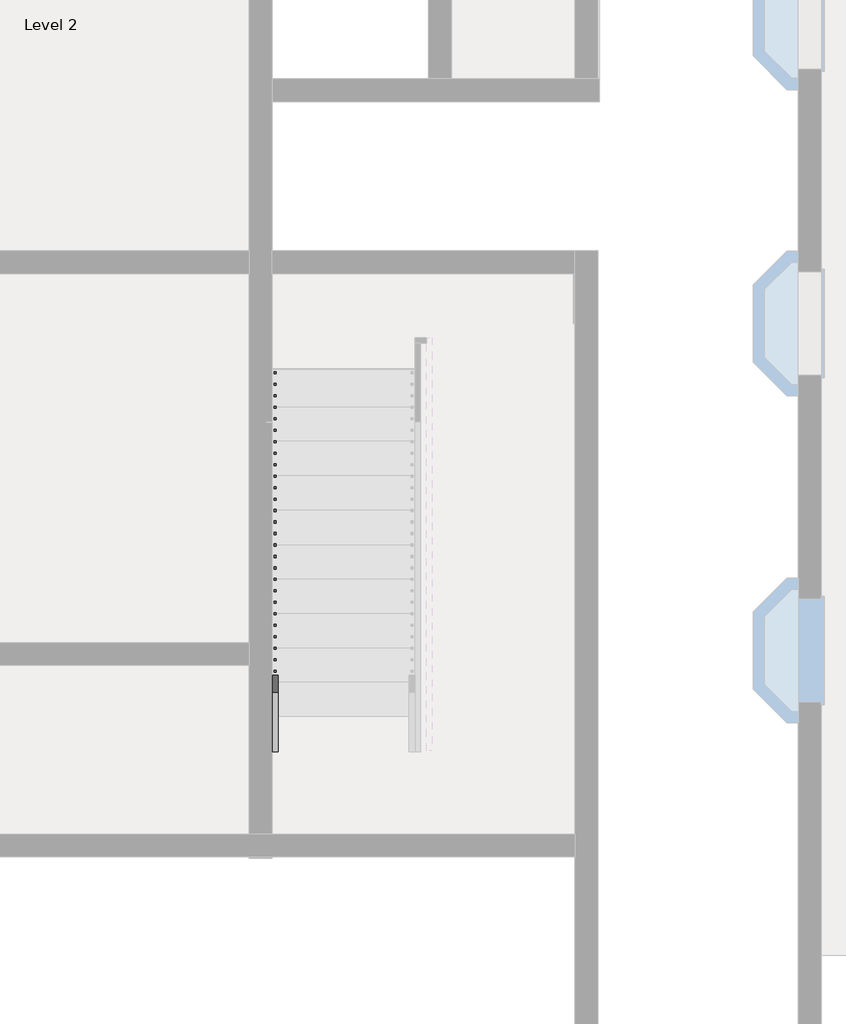
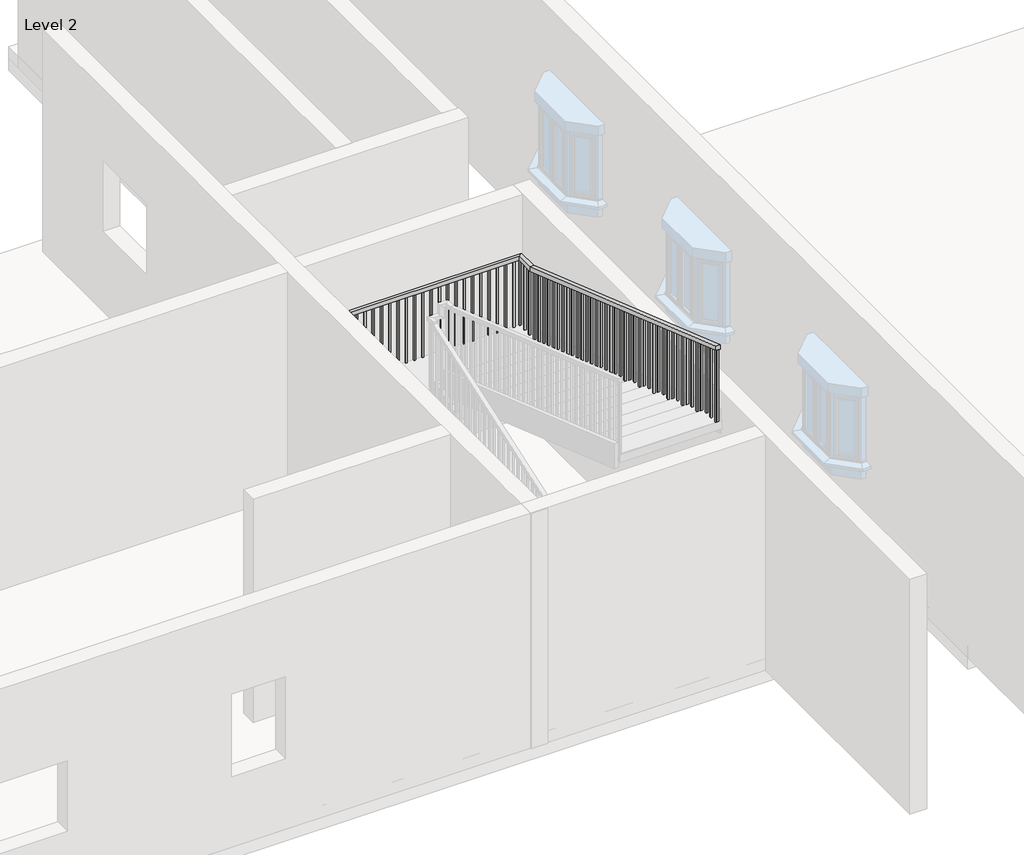
# One storey, part 8 of 14: 1 railing.
"""IFC4 building model written with IfcOpenShell, lengths in millimetres."""

from ifc_helpers import new_model, si_unit, frame, origin, place, context, project, spatial, polyline, outline, extrude, faceted_brep, element, save

model = new_model("IFC4")

# Units and contexts
model_context = context("Model", 3, world=origin())
ifc_project = project(units=[si_unit("LENGTHUNIT", "METRE", prefix="MILLI")], contexts=[model_context])

# Site, building, storey
site = spatial("IfcSite", under=ifc_project)
building = spatial("IfcBuilding", under=site)
storey = spatial("IfcBuildingStorey", under=building, Name="Level 2", Elevation=3048.0)

# Railing
placement = place(None, origin())
element("IfcRailing", 1, ObjectType="Handrail - Rectangular", at=placement, inside=storey, context=model_context, shape_type="SolidModel", body=[
    faceted_brep([(-3857.687215, -9955.5916506, 4067.9076923), (-3857.687215, -9955.5916506, 4014.1602476), (-3806.887215, -9955.5916506, 4014.1602476), (-3806.887215, -9955.5916506, 4067.9076923), (-3857.687215, -6291.6416506, 5334.0), (-3857.687215, -6283.1120276, 5283.2), (-3806.887215, -6283.1120276, 5283.2), (-3806.887215, -6291.6416506, 5334.0), (-3857.687215, -5713.7916506, 5334.0), (-3857.687215, -5713.7916506, 5283.2), (-3806.887215, -5764.5916506, 5283.2), (-3806.887215, -5764.5916506, 5334.0), (-1190.687215, -5713.7916506, 5334.0), (-1190.687215, -5713.7916506, 5283.2), (-1241.487215, -5764.5916506, 5283.2), (-1241.487215, -5764.5916506, 5334.0), (-1190.687215, -5986.8416506, 5334.0), (-1190.687215, -5995.3852679, 5283.2), (-1241.487215, -5995.3852679, 5283.2), (-1241.487215, -5986.8416506, 5334.0), (-1190.687215, -9949.2416506, 6705.6), (-1241.487215, -9949.2416506, 6705.6), (-1241.487215, -9949.2416506, 6651.842594), (-1190.687215, -9949.2416506, 6651.842594)], [[[0, 1, 2, 3]], [[1, 0, 4, 5]], [[2, 1, 5, 6]], [[3, 2, 6, 7]], [[0, 3, 7, 4]], [[5, 4, 8, 9]], [[6, 5, 9, 10]], [[7, 6, 10, 11]], [[4, 7, 11, 8]], [[9, 8, 12, 13]], [[10, 9, 13, 14]], [[11, 10, 14, 15]], [[8, 11, 15, 12]], [[13, 12, 16, 17]], [[14, 13, 17, 18]], [[15, 14, 18, 19]], [[12, 15, 19, 16]], [[20, 21, 22, 23]], [[17, 16, 20, 23]], [[18, 17, 23, 22]], [[19, 18, 22, 21]], [[16, 19, 21, 20]]]),
    extrude(outline(polyline([(-9895.2666506, 6633.1589402), (-9895.2666506, 5685.6923077), (-9914.3166506, 5685.6923077), (-9914.3166506, 6639.7531709), (-9895.2666506, 6633.1589402)])), frame((-1225.612215, 0.0, 0.0), z_axis=(1.0, 0.0, 0.0), x_axis=(0.0, 1.0, 0.0)), (0.0, 0.0, 1.0), 19.05),
    extrude(outline(polyline([(-9793.6666506, 6597.9897094), (-9793.6666506, 5685.6923077), (-9812.7166506, 5685.6923077), (-9812.7166506, 6604.5839402), (-9793.6666506, 6597.9897094)])), frame((-1225.612215, 0.0, 0.0), z_axis=(1.0, 0.0, 0.0), x_axis=(0.0, 1.0, 0.0)), (0.0, 0.0, 1.0), 19.05),
    extrude(outline(polyline([(-9692.0666506, 6562.8204786), (-9692.0666506, 5685.6923077), (-9711.1166506, 5685.6923077), (-9711.1166506, 6569.4147094), (-9692.0666506, 6562.8204786)])), frame((-1225.612215, 0.0, 0.0), z_axis=(1.0, 0.0, 0.0), x_axis=(0.0, 1.0, 0.0)), (0.0, 0.0, 1.0), 19.05),
    extrude(outline(polyline([(-9590.4666506, 6527.6512479), (-9590.4666506, 5580.1846154), (-9609.5166506, 5580.1846154), (-9609.5166506, 6534.2454786), (-9590.4666506, 6527.6512479)])), frame((-1225.612215, 0.0, 0.0), z_axis=(1.0, 0.0, 0.0), x_axis=(0.0, 1.0, 0.0)), (0.0, 0.0, 1.0), 19.05),
    extrude(outline(polyline([(-9488.8666506, 6492.4820171), (-9488.8666506, 5580.1846154), (-9507.9166506, 5580.1846154), (-9507.9166506, 6499.0762479), (-9488.8666506, 6492.4820171)])), frame((-1225.612215, 0.0, 0.0), z_axis=(1.0, 0.0, 0.0), x_axis=(0.0, 1.0, 0.0)), (0.0, 0.0, 1.0), 19.05),
    extrude(outline(polyline([(-9387.2666506, 6457.3127863), (-9387.2666506, 5580.1846154), (-9406.3166506, 5580.1846154), (-9406.3166506, 6463.9070171), (-9387.2666506, 6457.3127863)])), frame((-1225.612215, 0.0, 0.0), z_axis=(1.0, 0.0, 0.0), x_axis=(0.0, 1.0, 0.0)), (0.0, 0.0, 1.0), 19.05),
    extrude(outline(polyline([(-9285.6666506, 6422.1435556), (-9285.6666506, 5474.6769231), (-9304.7166506, 5474.6769231), (-9304.7166506, 6428.7377863), (-9285.6666506, 6422.1435556)])), frame((-1225.612215, 0.0, 0.0), z_axis=(1.0, 0.0, 0.0), x_axis=(0.0, 1.0, 0.0)), (0.0, 0.0, 1.0), 19.05),
    extrude(outline(polyline([(-9184.0666506, 6386.9743248), (-9184.0666506, 5474.6769231), (-9203.1166506, 5474.6769231), (-9203.1166506, 6393.5685556), (-9184.0666506, 6386.9743248)])), frame((-1225.612215, 0.0, 0.0), z_axis=(1.0, 0.0, 0.0), x_axis=(0.0, 1.0, 0.0)), (0.0, 0.0, 1.0), 19.05),
    extrude(outline(polyline([(-9082.4666506, 6351.805094), (-9082.4666506, 5474.6769231), (-9101.5166506, 5474.6769231), (-9101.5166506, 6358.3993248), (-9082.4666506, 6351.805094)])), frame((-1225.612215, 0.0, 0.0), z_axis=(1.0, 0.0, 0.0), x_axis=(0.0, 1.0, 0.0)), (0.0, 0.0, 1.0), 19.05),
    extrude(outline(polyline([(-8980.8666506, 6316.6358632), (-8980.8666506, 5369.1692308), (-8999.9166506, 5369.1692308), (-8999.9166506, 6323.230094), (-8980.8666506, 6316.6358632)])), frame((-1225.612215, 0.0, 0.0), z_axis=(1.0, 0.0, 0.0), x_axis=(0.0, 1.0, 0.0)), (0.0, 0.0, 1.0), 19.05),
    extrude(outline(polyline([(-8879.2666506, 6281.4666325), (-8879.2666506, 5369.1692308), (-8898.3166506, 5369.1692308), (-8898.3166506, 6288.0608632), (-8879.2666506, 6281.4666325)])), frame((-1225.612215, 0.0, 0.0), z_axis=(1.0, 0.0, 0.0), x_axis=(0.0, 1.0, 0.0)), (0.0, 0.0, 1.0), 19.05),
    extrude(outline(polyline([(-8777.6666506, 6246.2974017), (-8777.6666506, 5369.1692308), (-8796.7166506, 5369.1692308), (-8796.7166506, 6252.8916325), (-8777.6666506, 6246.2974017)])), frame((-1225.612215, 0.0, 0.0), z_axis=(1.0, 0.0, 0.0), x_axis=(0.0, 1.0, 0.0)), (0.0, 0.0, 1.0), 19.05),
    extrude(outline(polyline([(-8676.0666506, 6211.1281709), (-8676.0666506, 5263.6615385), (-8695.1166506, 5263.6615385), (-8695.1166506, 6217.7224017), (-8676.0666506, 6211.1281709)])), frame((-1225.612215, 0.0, 0.0), z_axis=(1.0, 0.0, 0.0), x_axis=(0.0, 1.0, 0.0)), (0.0, 0.0, 1.0), 19.05),
    extrude(outline(polyline([(-8574.4666506, 6175.9589402), (-8574.4666506, 5263.6615385), (-8593.5166506, 5263.6615385), (-8593.5166506, 6182.5531709), (-8574.4666506, 6175.9589402)])), frame((-1225.612215, 0.0, 0.0), z_axis=(1.0, 0.0, 0.0), x_axis=(0.0, 1.0, 0.0)), (0.0, 0.0, 1.0), 19.05),
    extrude(outline(polyline([(-8472.8666506, 6140.7897094), (-8472.8666506, 5263.6615385), (-8491.9166506, 5263.6615385), (-8491.9166506, 6147.3839402), (-8472.8666506, 6140.7897094)])), frame((-1225.612215, 0.0, 0.0), z_axis=(1.0, 0.0, 0.0), x_axis=(0.0, 1.0, 0.0)), (0.0, 0.0, 1.0), 19.05),
    extrude(outline(polyline([(-8371.2666506, 6105.6204786), (-8371.2666506, 5158.1538462), (-8390.3166506, 5158.1538462), (-8390.3166506, 6112.2147094), (-8371.2666506, 6105.6204786)])), frame((-1225.612215, 0.0, 0.0), z_axis=(1.0, 0.0, 0.0), x_axis=(0.0, 1.0, 0.0)), (0.0, 0.0, 1.0), 19.05),
    extrude(outline(polyline([(-8269.6666506, 6070.4512479), (-8269.6666506, 5158.1538462), (-8288.7166506, 5158.1538462), (-8288.7166506, 6077.0454786), (-8269.6666506, 6070.4512479)])), frame((-1225.612215, 0.0, 0.0), z_axis=(1.0, 0.0, 0.0), x_axis=(0.0, 1.0, 0.0)), (0.0, 0.0, 1.0), 19.05),
    extrude(outline(polyline([(-8168.0666506, 6035.2820171), (-8168.0666506, 5158.1538462), (-8187.1166506, 5158.1538462), (-8187.1166506, 6041.8762479), (-8168.0666506, 6035.2820171)])), frame((-1225.612215, 0.0, 0.0), z_axis=(1.0, 0.0, 0.0), x_axis=(0.0, 1.0, 0.0)), (0.0, 0.0, 1.0), 19.05),
    extrude(outline(polyline([(-8066.4666506, 6000.1127863), (-8066.4666506, 5052.6461538), (-8085.5166506, 5052.6461538), (-8085.5166506, 6006.7070171), (-8066.4666506, 6000.1127863)])), frame((-1225.612215, 0.0, 0.0), z_axis=(1.0, 0.0, 0.0), x_axis=(0.0, 1.0, 0.0)), (0.0, 0.0, 1.0), 19.05),
    extrude(outline(polyline([(-7964.8666506, 5964.9435556), (-7964.8666506, 5052.6461538), (-7983.9166506, 5052.6461538), (-7983.9166506, 5971.5377863), (-7964.8666506, 5964.9435556)])), frame((-1225.612215, 0.0, 0.0), z_axis=(1.0, 0.0, 0.0), x_axis=(0.0, 1.0, 0.0)), (0.0, 0.0, 1.0), 19.05),
    extrude(outline(polyline([(-7863.2666506, 5929.7743248), (-7863.2666506, 5052.6461538), (-7882.3166506, 5052.6461538), (-7882.3166506, 5936.3685556), (-7863.2666506, 5929.7743248)])), frame((-1225.612215, 0.0, 0.0), z_axis=(1.0, 0.0, 0.0), x_axis=(0.0, 1.0, 0.0)), (0.0, 0.0, 1.0), 19.05),
    extrude(outline(polyline([(-7761.6666506, 5894.605094), (-7761.6666506, 4947.1384615), (-7780.7166506, 4947.1384615), (-7780.7166506, 5901.1993248), (-7761.6666506, 5894.605094)])), frame((-1225.612215, 0.0, 0.0), z_axis=(1.0, 0.0, 0.0), x_axis=(0.0, 1.0, 0.0)), (0.0, 0.0, 1.0), 19.05),
    extrude(outline(polyline([(-7660.0666506, 5859.4358632), (-7660.0666506, 4947.1384615), (-7679.1166506, 4947.1384615), (-7679.1166506, 5866.030094), (-7660.0666506, 5859.4358632)])), frame((-1225.612215, 0.0, 0.0), z_axis=(1.0, 0.0, 0.0), x_axis=(0.0, 1.0, 0.0)), (0.0, 0.0, 1.0), 19.05),
    extrude(outline(polyline([(-7558.4666506, 5824.2666325), (-7558.4666506, 4947.1384615), (-7577.5166506, 4947.1384615), (-7577.5166506, 5830.8608632), (-7558.4666506, 5824.2666325)])), frame((-1225.612215, 0.0, 0.0), z_axis=(1.0, 0.0, 0.0), x_axis=(0.0, 1.0, 0.0)), (0.0, 0.0, 1.0), 19.05),
    extrude(outline(polyline([(-7456.8666506, 5789.0974017), (-7456.8666506, 4841.6307692), (-7475.9166506, 4841.6307692), (-7475.9166506, 5795.6916325), (-7456.8666506, 5789.0974017)])), frame((-1225.612215, 0.0, 0.0), z_axis=(1.0, 0.0, 0.0), x_axis=(0.0, 1.0, 0.0)), (0.0, 0.0, 1.0), 19.05),
    extrude(outline(polyline([(-7355.2666506, 5753.9281709), (-7355.2666506, 4841.6307692), (-7374.3166506, 4841.6307692), (-7374.3166506, 5760.5224017), (-7355.2666506, 5753.9281709)])), frame((-1225.612215, 0.0, 0.0), z_axis=(1.0, 0.0, 0.0), x_axis=(0.0, 1.0, 0.0)), (0.0, 0.0, 1.0), 19.05),
    extrude(outline(polyline([(-7253.6666506, 5718.7589402), (-7253.6666506, 4841.6307692), (-7272.7166506, 4841.6307692), (-7272.7166506, 5725.3531709), (-7253.6666506, 5718.7589402)])), frame((-1225.612215, 0.0, 0.0), z_axis=(1.0, 0.0, 0.0), x_axis=(0.0, 1.0, 0.0)), (0.0, 0.0, 1.0), 19.05),
    extrude(outline(polyline([(-7152.0666506, 5683.5897094), (-7152.0666506, 4736.1230769), (-7171.1166506, 4736.1230769), (-7171.1166506, 5690.1839402), (-7152.0666506, 5683.5897094)])), frame((-1225.612215, 0.0, 0.0), z_axis=(1.0, 0.0, 0.0), x_axis=(0.0, 1.0, 0.0)), (0.0, 0.0, 1.0), 19.05),
    extrude(outline(polyline([(-7050.4666506, 5648.4204786), (-7050.4666506, 4736.1230769), (-7069.5166506, 4736.1230769), (-7069.5166506, 5655.0147094), (-7050.4666506, 5648.4204786)])), frame((-1225.612215, 0.0, 0.0), z_axis=(1.0, 0.0, 0.0), x_axis=(0.0, 1.0, 0.0)), (0.0, 0.0, 1.0), 19.05),
    extrude(outline(polyline([(-6948.8666506, 5613.2512479), (-6948.8666506, 4736.1230769), (-6967.9166506, 4736.1230769), (-6967.9166506, 5619.8454786), (-6948.8666506, 5613.2512479)])), frame((-1225.612215, 0.0, 0.0), z_axis=(1.0, 0.0, 0.0), x_axis=(0.0, 1.0, 0.0)), (0.0, 0.0, 1.0), 19.05),
    extrude(outline(polyline([(-6847.2666506, 5578.0820171), (-6847.2666506, 4630.6153846), (-6866.3166506, 4630.6153846), (-6866.3166506, 5584.6762479), (-6847.2666506, 5578.0820171)])), frame((-1225.612215, 0.0, 0.0), z_axis=(1.0, 0.0, 0.0), x_axis=(0.0, 1.0, 0.0)), (0.0, 0.0, 1.0), 19.05),
    extrude(outline(polyline([(-6745.6666506, 5542.9127863), (-6745.6666506, 4630.6153846), (-6764.7166506, 4630.6153846), (-6764.7166506, 5549.5070171), (-6745.6666506, 5542.9127863)])), frame((-1225.612215, 0.0, 0.0), z_axis=(1.0, 0.0, 0.0), x_axis=(0.0, 1.0, 0.0)), (0.0, 0.0, 1.0), 19.05),
    extrude(outline(polyline([(-6644.0666506, 5507.7435556), (-6644.0666506, 4630.6153846), (-6663.1166506, 4630.6153846), (-6663.1166506, 5514.3377863), (-6644.0666506, 5507.7435556)])), frame((-1225.612215, 0.0, 0.0), z_axis=(1.0, 0.0, 0.0), x_axis=(0.0, 1.0, 0.0)), (0.0, 0.0, 1.0), 19.05),
    extrude(outline(polyline([(-6542.4666506, 5472.5743248), (-6542.4666506, 4525.1076923), (-6561.5166506, 4525.1076923), (-6561.5166506, 5479.1685556), (-6542.4666506, 5472.5743248)])), frame((-1225.612215, 0.0, 0.0), z_axis=(1.0, 0.0, 0.0), x_axis=(0.0, 1.0, 0.0)), (0.0, 0.0, 1.0), 19.05),
    extrude(outline(polyline([(-6440.8666506, 5437.405094), (-6440.8666506, 4525.1076923), (-6459.9166506, 4525.1076923), (-6459.9166506, 5443.9993248), (-6440.8666506, 5437.405094)])), frame((-1225.612215, 0.0, 0.0), z_axis=(1.0, 0.0, 0.0), x_axis=(0.0, 1.0, 0.0)), (0.0, 0.0, 1.0), 19.05),
    extrude(outline(polyline([(-6339.2666506, 5402.2358632), (-6339.2666506, 4525.1076923), (-6358.3166506, 4525.1076923), (-6358.3166506, 5408.830094), (-6339.2666506, 5402.2358632)])), frame((-1225.612215, 0.0, 0.0), z_axis=(1.0, 0.0, 0.0), x_axis=(0.0, 1.0, 0.0)), (0.0, 0.0, 1.0), 19.05),
    extrude(outline(polyline([(-6237.6666506, 5367.0666325), (-6237.6666506, 4419.6), (-6256.7166506, 4419.6), (-6256.7166506, 5373.6608632), (-6237.6666506, 5367.0666325)])), frame((-1225.612215, 0.0, 0.0), z_axis=(1.0, 0.0, 0.0), x_axis=(0.0, 1.0, 0.0)), (0.0, 0.0, 1.0), 19.05),
    extrude(outline(polyline([(-6136.0666506, 5331.8974017), (-6136.0666506, 4419.6), (-6155.1166506, 4419.6), (-6155.1166506, 5338.4916325), (-6136.0666506, 5331.8974017)])), frame((-1225.612215, 0.0, 0.0), z_axis=(1.0, 0.0, 0.0), x_axis=(0.0, 1.0, 0.0)), (0.0, 0.0, 1.0), 19.05),
    extrude(outline(polyline([(-6034.4666506, 5296.7281709), (-6034.4666506, 4419.6), (-6053.5166506, 4419.6), (-6053.5166506, 5303.3224017), (-6034.4666506, 5296.7281709)])), frame((-1225.612215, 0.0, 0.0), z_axis=(1.0, 0.0, 0.0), x_axis=(0.0, 1.0, 0.0)), (0.0, 0.0, 1.0), 19.05),
    extrude(outline(polyline([(-1206.562215, -5932.8666506), (-1206.562215, -5951.9166506), (-1225.612215, -5951.9166506), (-1225.612215, -5932.8666506), (-1206.562215, -5932.8666506)])), frame((0.0, 0.0, 4419.6), z_axis=(0.0, 0.0, 1.0), x_axis=(1.0, 0.0, 0.0)), (0.0, 0.0, 1.0), 863.6),
    extrude(outline(polyline([(-1206.562215, -5831.2666506), (-1206.562215, -5850.3166506), (-1225.612215, -5850.3166506), (-1225.612215, -5831.2666506), (-1206.562215, -5831.2666506)])), frame((0.0, 0.0, 4419.6), z_axis=(0.0, 0.0, 1.0), x_axis=(1.0, 0.0, 0.0)), (0.0, 0.0, 1.0), 863.6),
    extrude(outline(polyline([(-1301.812215, -5729.6666506), (-1282.762215, -5729.6666506), (-1282.762215, -5748.7166506), (-1301.812215, -5748.7166506), (-1301.812215, -5729.6666506)])), frame((0.0, 0.0, 4419.6), z_axis=(0.0, 0.0, 1.0), x_axis=(1.0, 0.0, 0.0)), (0.0, 0.0, 1.0), 863.6),
    extrude(outline(polyline([(-1403.412215, -5729.6666506), (-1384.362215, -5729.6666506), (-1384.362215, -5748.7166506), (-1403.412215, -5748.7166506), (-1403.412215, -5729.6666506)])), frame((0.0, 0.0, 4419.6), z_axis=(0.0, 0.0, 1.0), x_axis=(1.0, 0.0, 0.0)), (0.0, 0.0, 1.0), 863.6),
    extrude(outline(polyline([(-1505.012215, -5729.6666506), (-1485.962215, -5729.6666506), (-1485.962215, -5748.7166506), (-1505.012215, -5748.7166506), (-1505.012215, -5729.6666506)])), frame((0.0, 0.0, 4419.6), z_axis=(0.0, 0.0, 1.0), x_axis=(1.0, 0.0, 0.0)), (0.0, 0.0, 1.0), 863.6),
    extrude(outline(polyline([(-1606.612215, -5729.6666506), (-1587.562215, -5729.6666506), (-1587.562215, -5748.7166506), (-1606.612215, -5748.7166506), (-1606.612215, -5729.6666506)])), frame((0.0, 0.0, 4419.6), z_axis=(0.0, 0.0, 1.0), x_axis=(1.0, 0.0, 0.0)), (0.0, 0.0, 1.0), 863.6),
    extrude(outline(polyline([(-1708.212215, -5729.6666506), (-1689.162215, -5729.6666506), (-1689.162215, -5748.7166506), (-1708.212215, -5748.7166506), (-1708.212215, -5729.6666506)])), frame((0.0, 0.0, 4419.6), z_axis=(0.0, 0.0, 1.0), x_axis=(1.0, 0.0, 0.0)), (0.0, 0.0, 1.0), 863.6),
    extrude(outline(polyline([(-1809.812215, -5729.6666506), (-1790.762215, -5729.6666506), (-1790.762215, -5748.7166506), (-1809.812215, -5748.7166506), (-1809.812215, -5729.6666506)])), frame((0.0, 0.0, 4419.6), z_axis=(0.0, 0.0, 1.0), x_axis=(1.0, 0.0, 0.0)), (0.0, 0.0, 1.0), 863.6),
    extrude(outline(polyline([(-1911.412215, -5729.6666506), (-1892.362215, -5729.6666506), (-1892.362215, -5748.7166506), (-1911.412215, -5748.7166506), (-1911.412215, -5729.6666506)])), frame((0.0, 0.0, 4419.6), z_axis=(0.0, 0.0, 1.0), x_axis=(1.0, 0.0, 0.0)), (0.0, 0.0, 1.0), 863.6),
    extrude(outline(polyline([(-2013.012215, -5729.6666506), (-1993.962215, -5729.6666506), (-1993.962215, -5748.7166506), (-2013.012215, -5748.7166506), (-2013.012215, -5729.6666506)])), frame((0.0, 0.0, 4419.6), z_axis=(0.0, 0.0, 1.0), x_axis=(1.0, 0.0, 0.0)), (0.0, 0.0, 1.0), 863.6),
    extrude(outline(polyline([(-2114.612215, -5729.6666506), (-2095.562215, -5729.6666506), (-2095.562215, -5748.7166506), (-2114.612215, -5748.7166506), (-2114.612215, -5729.6666506)])), frame((0.0, 0.0, 4419.6), z_axis=(0.0, 0.0, 1.0), x_axis=(1.0, 0.0, 0.0)), (0.0, 0.0, 1.0), 863.6),
    extrude(outline(polyline([(-2216.212215, -5729.6666506), (-2197.162215, -5729.6666506), (-2197.162215, -5748.7166506), (-2216.212215, -5748.7166506), (-2216.212215, -5729.6666506)])), frame((0.0, 0.0, 4419.6), z_axis=(0.0, 0.0, 1.0), x_axis=(1.0, 0.0, 0.0)), (0.0, 0.0, 1.0), 863.6),
    extrude(outline(polyline([(-2317.812215, -5729.6666506), (-2298.762215, -5729.6666506), (-2298.762215, -5748.7166506), (-2317.812215, -5748.7166506), (-2317.812215, -5729.6666506)])), frame((0.0, 0.0, 4419.6), z_axis=(0.0, 0.0, 1.0), x_axis=(1.0, 0.0, 0.0)), (0.0, 0.0, 1.0), 863.6),
    extrude(outline(polyline([(-2419.412215, -5729.6666506), (-2400.362215, -5729.6666506), (-2400.362215, -5748.7166506), (-2419.412215, -5748.7166506), (-2419.412215, -5729.6666506)])), frame((0.0, 0.0, 4419.6), z_axis=(0.0, 0.0, 1.0), x_axis=(1.0, 0.0, 0.0)), (0.0, 0.0, 1.0), 863.6),
    extrude(outline(polyline([(-2521.012215, -5729.6666506), (-2501.962215, -5729.6666506), (-2501.962215, -5748.7166506), (-2521.012215, -5748.7166506), (-2521.012215, -5729.6666506)])), frame((0.0, 0.0, 4419.6), z_axis=(0.0, 0.0, 1.0), x_axis=(1.0, 0.0, 0.0)), (0.0, 0.0, 1.0), 863.6),
    extrude(outline(polyline([(-2622.612215, -5729.6666506), (-2603.562215, -5729.6666506), (-2603.562215, -5748.7166506), (-2622.612215, -5748.7166506), (-2622.612215, -5729.6666506)])), frame((0.0, 0.0, 4419.6), z_axis=(0.0, 0.0, 1.0), x_axis=(1.0, 0.0, 0.0)), (0.0, 0.0, 1.0), 863.6),
    extrude(outline(polyline([(-2724.212215, -5729.6666506), (-2705.162215, -5729.6666506), (-2705.162215, -5748.7166506), (-2724.212215, -5748.7166506), (-2724.212215, -5729.6666506)])), frame((0.0, 0.0, 4419.6), z_axis=(0.0, 0.0, 1.0), x_axis=(1.0, 0.0, 0.0)), (0.0, 0.0, 1.0), 863.6),
    extrude(outline(polyline([(-2825.812215, -5729.6666506), (-2806.762215, -5729.6666506), (-2806.762215, -5748.7166506), (-2825.812215, -5748.7166506), (-2825.812215, -5729.6666506)])), frame((0.0, 0.0, 4419.6), z_axis=(0.0, 0.0, 1.0), x_axis=(1.0, 0.0, 0.0)), (0.0, 0.0, 1.0), 863.6),
    extrude(outline(polyline([(-2927.412215, -5729.6666506), (-2908.362215, -5729.6666506), (-2908.362215, -5748.7166506), (-2927.412215, -5748.7166506), (-2927.412215, -5729.6666506)])), frame((0.0, 0.0, 4419.6), z_axis=(0.0, 0.0, 1.0), x_axis=(1.0, 0.0, 0.0)), (0.0, 0.0, 1.0), 863.6),
    extrude(outline(polyline([(-3029.012215, -5729.6666506), (-3009.962215, -5729.6666506), (-3009.962215, -5748.7166506), (-3029.012215, -5748.7166506), (-3029.012215, -5729.6666506)])), frame((0.0, 0.0, 4419.6), z_axis=(0.0, 0.0, 1.0), x_axis=(1.0, 0.0, 0.0)), (0.0, 0.0, 1.0), 863.6),
    extrude(outline(polyline([(-3130.612215, -5729.6666506), (-3111.562215, -5729.6666506), (-3111.562215, -5748.7166506), (-3130.612215, -5748.7166506), (-3130.612215, -5729.6666506)])), frame((0.0, 0.0, 4419.6), z_axis=(0.0, 0.0, 1.0), x_axis=(1.0, 0.0, 0.0)), (0.0, 0.0, 1.0), 863.6),
    extrude(outline(polyline([(-3232.212215, -5729.6666506), (-3213.162215, -5729.6666506), (-3213.162215, -5748.7166506), (-3232.212215, -5748.7166506), (-3232.212215, -5729.6666506)])), frame((0.0, 0.0, 4419.6), z_axis=(0.0, 0.0, 1.0), x_axis=(1.0, 0.0, 0.0)), (0.0, 0.0, 1.0), 863.6),
    extrude(outline(polyline([(-3333.812215, -5729.6666506), (-3314.762215, -5729.6666506), (-3314.762215, -5748.7166506), (-3333.812215, -5748.7166506), (-3333.812215, -5729.6666506)])), frame((0.0, 0.0, 4419.6), z_axis=(0.0, 0.0, 1.0), x_axis=(1.0, 0.0, 0.0)), (0.0, 0.0, 1.0), 863.6),
    extrude(outline(polyline([(-3435.412215, -5729.6666506), (-3416.362215, -5729.6666506), (-3416.362215, -5748.7166506), (-3435.412215, -5748.7166506), (-3435.412215, -5729.6666506)])), frame((0.0, 0.0, 4419.6), z_axis=(0.0, 0.0, 1.0), x_axis=(1.0, 0.0, 0.0)), (0.0, 0.0, 1.0), 863.6),
    extrude(outline(polyline([(-3537.012215, -5729.6666506), (-3517.962215, -5729.6666506), (-3517.962215, -5748.7166506), (-3537.012215, -5748.7166506), (-3537.012215, -5729.6666506)])), frame((0.0, 0.0, 4419.6), z_axis=(0.0, 0.0, 1.0), x_axis=(1.0, 0.0, 0.0)), (0.0, 0.0, 1.0), 863.6),
    extrude(outline(polyline([(-3638.612215, -5729.6666506), (-3619.562215, -5729.6666506), (-3619.562215, -5748.7166506), (-3638.612215, -5748.7166506), (-3638.612215, -5729.6666506)])), frame((0.0, 0.0, 4419.6), z_axis=(0.0, 0.0, 1.0), x_axis=(1.0, 0.0, 0.0)), (0.0, 0.0, 1.0), 863.6),
    extrude(outline(polyline([(-3740.212215, -5729.6666506), (-3721.162215, -5729.6666506), (-3721.162215, -5748.7166506), (-3740.212215, -5748.7166506), (-3740.212215, -5729.6666506)])), frame((0.0, 0.0, 4419.6), z_axis=(0.0, 0.0, 1.0), x_axis=(1.0, 0.0, 0.0)), (0.0, 0.0, 1.0), 863.6),
    extrude(outline(polyline([(-3841.812215, -5799.5166506), (-3841.812215, -5780.4666506), (-3822.762215, -5780.4666506), (-3822.762215, -5799.5166506), (-3841.812215, -5799.5166506)])), frame((0.0, 0.0, 4419.6), z_axis=(0.0, 0.0, 1.0), x_axis=(1.0, 0.0, 0.0)), (0.0, 0.0, 1.0), 863.6),
    extrude(outline(polyline([(-3841.812215, -5901.1166506), (-3841.812215, -5882.0666506), (-3822.762215, -5882.0666506), (-3822.762215, -5901.1166506), (-3841.812215, -5901.1166506)])), frame((0.0, 0.0, 4419.6), z_axis=(0.0, 0.0, 1.0), x_axis=(1.0, 0.0, 0.0)), (0.0, 0.0, 1.0), 863.6),
    extrude(outline(polyline([(-3841.812215, -6002.7166506), (-3841.812215, -5983.6666506), (-3822.762215, -5983.6666506), (-3822.762215, -6002.7166506), (-3841.812215, -6002.7166506)])), frame((0.0, 0.0, 4419.6), z_axis=(0.0, 0.0, 1.0), x_axis=(1.0, 0.0, 0.0)), (0.0, 0.0, 1.0), 863.6),
    extrude(outline(polyline([(-3841.812215, -6104.3166506), (-3841.812215, -6085.2666506), (-3822.762215, -6085.2666506), (-3822.762215, -6104.3166506), (-3841.812215, -6104.3166506)])), frame((0.0, 0.0, 4419.6), z_axis=(0.0, 0.0, 1.0), x_axis=(1.0, 0.0, 0.0)), (0.0, 0.0, 1.0), 863.6),
    extrude(outline(polyline([(-3841.812215, -6205.9166506), (-3841.812215, -6186.8666506), (-3822.762215, -6186.8666506), (-3822.762215, -6205.9166506), (-3841.812215, -6205.9166506)])), frame((0.0, 0.0, 4419.6), z_axis=(0.0, 0.0, 1.0), x_axis=(1.0, 0.0, 0.0)), (0.0, 0.0, 1.0), 863.6),
    extrude(outline(polyline([(-6288.4666506, 5281.349689), (-6288.4666506, 4314.0923077), (-6307.5166506, 4314.0923077), (-6307.5166506, 5274.7668867), (-6288.4666506, 5281.349689)])), frame((-3841.812215, 0.0, 0.0), z_axis=(1.0, 0.0, 0.0), x_axis=(0.0, 1.0, 0.0)), (0.0, 0.0, 1.0), 19.05),
    extrude(outline(polyline([(-6390.0666506, 5246.2414101), (-6390.0666506, 4314.0923077), (-6409.1166506, 4314.0923077), (-6409.1166506, 5239.6586078), (-6390.0666506, 5246.2414101)])), frame((-3841.812215, 0.0, 0.0), z_axis=(1.0, 0.0, 0.0), x_axis=(0.0, 1.0, 0.0)), (0.0, 0.0, 1.0), 19.05),
    extrude(outline(polyline([(-6491.6666506, 5211.1331312), (-6491.6666506, 4314.0923077), (-6510.7166506, 4314.0923077), (-6510.7166506, 5204.5503289), (-6491.6666506, 5211.1331312)])), frame((-3841.812215, 0.0, 0.0), z_axis=(1.0, 0.0, 0.0), x_axis=(0.0, 1.0, 0.0)), (0.0, 0.0, 1.0), 19.05),
    extrude(outline(polyline([(-6593.2666506, 5176.0248523), (-6593.2666506, 4208.5846154), (-6612.3166506, 4208.5846154), (-6612.3166506, 5169.44205), (-6593.2666506, 5176.0248523)])), frame((-3841.812215, 0.0, 0.0), z_axis=(1.0, 0.0, 0.0), x_axis=(0.0, 1.0, 0.0)), (0.0, 0.0, 1.0), 19.05),
    extrude(outline(polyline([(-6694.8666506, 5140.9165734), (-6694.8666506, 4208.5846154), (-6713.9166506, 4208.5846154), (-6713.9166506, 5134.3337711), (-6694.8666506, 5140.9165734)])), frame((-3841.812215, 0.0, 0.0), z_axis=(1.0, 0.0, 0.0), x_axis=(0.0, 1.0, 0.0)), (0.0, 0.0, 1.0), 19.05),
    extrude(outline(polyline([(-6796.4666506, 5105.8082945), (-6796.4666506, 4208.5846154), (-6815.5166506, 4208.5846154), (-6815.5166506, 5099.2254922), (-6796.4666506, 5105.8082945)])), frame((-3841.812215, 0.0, 0.0), z_axis=(1.0, 0.0, 0.0), x_axis=(0.0, 1.0, 0.0)), (0.0, 0.0, 1.0), 19.05),
    extrude(outline(polyline([(-6898.0666506, 5070.7000156), (-6898.0666506, 4103.0769231), (-6917.1166506, 4103.0769231), (-6917.1166506, 5064.1172133), (-6898.0666506, 5070.7000156)])), frame((-3841.812215, 0.0, 0.0), z_axis=(1.0, 0.0, 0.0), x_axis=(0.0, 1.0, 0.0)), (0.0, 0.0, 1.0), 19.05),
    extrude(outline(polyline([(-6999.6666506, 5035.5917367), (-6999.6666506, 4103.0769231), (-7018.7166506, 4103.0769231), (-7018.7166506, 5029.0089344), (-6999.6666506, 5035.5917367)])), frame((-3841.812215, 0.0, 0.0), z_axis=(1.0, 0.0, 0.0), x_axis=(0.0, 1.0, 0.0)), (0.0, 0.0, 1.0), 19.05),
    extrude(outline(polyline([(-7101.2666506, 5000.4834578), (-7101.2666506, 4103.0769231), (-7120.3166506, 4103.0769231), (-7120.3166506, 4993.9006556), (-7101.2666506, 5000.4834578)])), frame((-3841.812215, 0.0, 0.0), z_axis=(1.0, 0.0, 0.0), x_axis=(0.0, 1.0, 0.0)), (0.0, 0.0, 1.0), 19.05),
    extrude(outline(polyline([(-7202.8666506, 4965.3751789), (-7202.8666506, 3997.5692308), (-7221.9166506, 3997.5692308), (-7221.9166506, 4958.7923767), (-7202.8666506, 4965.3751789)])), frame((-3841.812215, 0.0, 0.0), z_axis=(1.0, 0.0, 0.0), x_axis=(0.0, 1.0, 0.0)), (0.0, 0.0, 1.0), 19.05),
    extrude(outline(polyline([(-7304.4666506, 4930.2669001), (-7304.4666506, 3997.5692308), (-7323.5166506, 3997.5692308), (-7323.5166506, 4923.6840978), (-7304.4666506, 4930.2669001)])), frame((-3841.812215, 0.0, 0.0), z_axis=(1.0, 0.0, 0.0), x_axis=(0.0, 1.0, 0.0)), (0.0, 0.0, 1.0), 19.05),
    extrude(outline(polyline([(-7406.0666506, 4895.1586212), (-7406.0666506, 3997.5692308), (-7425.1166506, 3997.5692308), (-7425.1166506, 4888.5758189), (-7406.0666506, 4895.1586212)])), frame((-3841.812215, 0.0, 0.0), z_axis=(1.0, 0.0, 0.0), x_axis=(0.0, 1.0, 0.0)), (0.0, 0.0, 1.0), 19.05),
    extrude(outline(polyline([(-7507.6666506, 4860.0503423), (-7507.6666506, 3892.0615385), (-7526.7166506, 3892.0615385), (-7526.7166506, 4853.46754), (-7507.6666506, 4860.0503423)])), frame((-3841.812215, 0.0, 0.0), z_axis=(1.0, 0.0, 0.0), x_axis=(0.0, 1.0, 0.0)), (0.0, 0.0, 1.0), 19.05),
    extrude(outline(polyline([(-7609.2666506, 4824.9420634), (-7609.2666506, 3892.0615385), (-7628.3166506, 3892.0615385), (-7628.3166506, 4818.3592611), (-7609.2666506, 4824.9420634)])), frame((-3841.812215, 0.0, 0.0), z_axis=(1.0, 0.0, 0.0), x_axis=(0.0, 1.0, 0.0)), (0.0, 0.0, 1.0), 19.05),
    extrude(outline(polyline([(-7710.8666506, 4789.8337845), (-7710.8666506, 3892.0615385), (-7729.9166506, 3892.0615385), (-7729.9166506, 4783.2509822), (-7710.8666506, 4789.8337845)])), frame((-3841.812215, 0.0, 0.0), z_axis=(1.0, 0.0, 0.0), x_axis=(0.0, 1.0, 0.0)), (0.0, 0.0, 1.0), 19.05),
    extrude(outline(polyline([(-7812.4666506, 4754.7255056), (-7812.4666506, 3786.5538462), (-7831.5166506, 3786.5538462), (-7831.5166506, 4748.1427033), (-7812.4666506, 4754.7255056)])), frame((-3841.812215, 0.0, 0.0), z_axis=(1.0, 0.0, 0.0), x_axis=(0.0, 1.0, 0.0)), (0.0, 0.0, 1.0), 19.05),
    extrude(outline(polyline([(-7914.0666506, 4719.6172267), (-7914.0666506, 3786.5538462), (-7933.1166506, 3786.5538462), (-7933.1166506, 4713.0344244), (-7914.0666506, 4719.6172267)])), frame((-3841.812215, 0.0, 0.0), z_axis=(1.0, 0.0, 0.0), x_axis=(0.0, 1.0, 0.0)), (0.0, 0.0, 1.0), 19.05),
    extrude(outline(polyline([(-8015.6666506, 4684.5089478), (-8015.6666506, 3786.5538462), (-8034.7166506, 3786.5538462), (-8034.7166506, 4677.9261455), (-8015.6666506, 4684.5089478)])), frame((-3841.812215, 0.0, 0.0), z_axis=(1.0, 0.0, 0.0), x_axis=(0.0, 1.0, 0.0)), (0.0, 0.0, 1.0), 19.05),
    extrude(outline(polyline([(-8117.2666506, 4649.4006689), (-8117.2666506, 3681.0461538), (-8136.3166506, 3681.0461538), (-8136.3166506, 4642.8178666), (-8117.2666506, 4649.4006689)])), frame((-3841.812215, 0.0, 0.0), z_axis=(1.0, 0.0, 0.0), x_axis=(0.0, 1.0, 0.0)), (0.0, 0.0, 1.0), 19.05),
    extrude(outline(polyline([(-8218.8666506, 4614.29239), (-8218.8666506, 3681.0461538), (-8237.9166506, 3681.0461538), (-8237.9166506, 4607.7095877), (-8218.8666506, 4614.29239)])), frame((-3841.812215, 0.0, 0.0), z_axis=(1.0, 0.0, 0.0), x_axis=(0.0, 1.0, 0.0)), (0.0, 0.0, 1.0), 19.05),
    extrude(outline(polyline([(-8320.4666506, 4579.1841111), (-8320.4666506, 3681.0461538), (-8339.5166506, 3681.0461538), (-8339.5166506, 4572.6013088), (-8320.4666506, 4579.1841111)])), frame((-3841.812215, 0.0, 0.0), z_axis=(1.0, 0.0, 0.0), x_axis=(0.0, 1.0, 0.0)), (0.0, 0.0, 1.0), 19.05),
    extrude(outline(polyline([(-8422.0666506, 4544.0758322), (-8422.0666506, 3575.5384615), (-8441.1166506, 3575.5384615), (-8441.1166506, 4537.4930299), (-8422.0666506, 4544.0758322)])), frame((-3841.812215, 0.0, 0.0), z_axis=(1.0, 0.0, 0.0), x_axis=(0.0, 1.0, 0.0)), (0.0, 0.0, 1.0), 19.05),
    extrude(outline(polyline([(-8523.6666506, 4508.9675533), (-8523.6666506, 3575.5384615), (-8542.7166506, 3575.5384615), (-8542.7166506, 4502.384751), (-8523.6666506, 4508.9675533)])), frame((-3841.812215, 0.0, 0.0), z_axis=(1.0, 0.0, 0.0), x_axis=(0.0, 1.0, 0.0)), (0.0, 0.0, 1.0), 19.05),
    extrude(outline(polyline([(-8625.2666506, 4473.8592744), (-8625.2666506, 3575.5384615), (-8644.3166506, 3575.5384615), (-8644.3166506, 4467.2764721), (-8625.2666506, 4473.8592744)])), frame((-3841.812215, 0.0, 0.0), z_axis=(1.0, 0.0, 0.0), x_axis=(0.0, 1.0, 0.0)), (0.0, 0.0, 1.0), 19.05),
    extrude(outline(polyline([(-8726.8666506, 4438.7509955), (-8726.8666506, 3470.0307692), (-8745.9166506, 3470.0307692), (-8745.9166506, 4432.1681932), (-8726.8666506, 4438.7509955)])), frame((-3841.812215, 0.0, 0.0), z_axis=(1.0, 0.0, 0.0), x_axis=(0.0, 1.0, 0.0)), (0.0, 0.0, 1.0), 19.05),
    extrude(outline(polyline([(-8828.4666506, 4403.6427166), (-8828.4666506, 3470.0307692), (-8847.5166506, 3470.0307692), (-8847.5166506, 4397.0599143), (-8828.4666506, 4403.6427166)])), frame((-3841.812215, 0.0, 0.0), z_axis=(1.0, 0.0, 0.0), x_axis=(0.0, 1.0, 0.0)), (0.0, 0.0, 1.0), 19.05),
    extrude(outline(polyline([(-8930.0666506, 4368.5344377), (-8930.0666506, 3470.0307692), (-8949.1166506, 3470.0307692), (-8949.1166506, 4361.9516354), (-8930.0666506, 4368.5344377)])), frame((-3841.812215, 0.0, 0.0), z_axis=(1.0, 0.0, 0.0), x_axis=(0.0, 1.0, 0.0)), (0.0, 0.0, 1.0), 19.05),
    extrude(outline(polyline([(-9031.6666506, 4333.4261588), (-9031.6666506, 3364.5230769), (-9050.7166506, 3364.5230769), (-9050.7166506, 4326.8433565), (-9031.6666506, 4333.4261588)])), frame((-3841.812215, 0.0, 0.0), z_axis=(1.0, 0.0, 0.0), x_axis=(0.0, 1.0, 0.0)), (0.0, 0.0, 1.0), 19.05),
    extrude(outline(polyline([(-9133.2666506, 4298.3178799), (-9133.2666506, 3364.5230769), (-9152.3166506, 3364.5230769), (-9152.3166506, 4291.7350776), (-9133.2666506, 4298.3178799)])), frame((-3841.812215, 0.0, 0.0), z_axis=(1.0, 0.0, 0.0), x_axis=(0.0, 1.0, 0.0)), (0.0, 0.0, 1.0), 19.05),
    extrude(outline(polyline([(-9234.8666506, 4263.209601), (-9234.8666506, 3364.5230769), (-9253.9166506, 3364.5230769), (-9253.9166506, 4256.6267987), (-9234.8666506, 4263.209601)])), frame((-3841.812215, 0.0, 0.0), z_axis=(1.0, 0.0, 0.0), x_axis=(0.0, 1.0, 0.0)), (0.0, 0.0, 1.0), 19.05),
    extrude(outline(polyline([(-9336.4666506, 4228.1013221), (-9336.4666506, 3259.0153846), (-9355.5166506, 3259.0153846), (-9355.5166506, 4221.5185198), (-9336.4666506, 4228.1013221)])), frame((-3841.812215, 0.0, 0.0), z_axis=(1.0, 0.0, 0.0), x_axis=(0.0, 1.0, 0.0)), (0.0, 0.0, 1.0), 19.05),
    extrude(outline(polyline([(-9438.0666506, 4192.9930432), (-9438.0666506, 3259.0153846), (-9457.1166506, 3259.0153846), (-9457.1166506, 4186.4102409), (-9438.0666506, 4192.9930432)])), frame((-3841.812215, 0.0, 0.0), z_axis=(1.0, 0.0, 0.0), x_axis=(0.0, 1.0, 0.0)), (0.0, 0.0, 1.0), 19.05),
    extrude(outline(polyline([(-9539.6666506, 4157.8847643), (-9539.6666506, 3259.0153846), (-9558.7166506, 3259.0153846), (-9558.7166506, 4151.301962), (-9539.6666506, 4157.8847643)])), frame((-3841.812215, 0.0, 0.0), z_axis=(1.0, 0.0, 0.0), x_axis=(0.0, 1.0, 0.0)), (0.0, 0.0, 1.0), 19.05),
    extrude(outline(polyline([(-9641.2666506, 4122.7764854), (-9641.2666506, 3153.5076923), (-9660.3166506, 3153.5076923), (-9660.3166506, 4116.1936831), (-9641.2666506, 4122.7764854)])), frame((-3841.812215, 0.0, 0.0), z_axis=(1.0, 0.0, 0.0), x_axis=(0.0, 1.0, 0.0)), (0.0, 0.0, 1.0), 19.05),
    extrude(outline(polyline([(-9742.8666506, 4087.6682065), (-9742.8666506, 3153.5076923), (-9761.9166506, 3153.5076923), (-9761.9166506, 4081.0854043), (-9742.8666506, 4087.6682065)])), frame((-3841.812215, 0.0, 0.0), z_axis=(1.0, 0.0, 0.0), x_axis=(0.0, 1.0, 0.0)), (0.0, 0.0, 1.0), 19.05),
    extrude(outline(polyline([(-9844.4666506, 4052.5599277), (-9844.4666506, 3153.5076923), (-9863.5166506, 3153.5076923), (-9863.5166506, 4045.9771254), (-9844.4666506, 4052.5599277)])), frame((-3841.812215, 0.0, 0.0), z_axis=(1.0, 0.0, 0.0), x_axis=(0.0, 1.0, 0.0)), (0.0, 0.0, 1.0), 19.05),
    extrude(outline(polyline([(-1225.612215, -5729.6666506), (-1206.562215, -5729.6666506), (-1206.562215, -5748.7166506), (-1225.612215, -5748.7166506), (-1225.612215, -5729.6666506)])), frame((0.0, 0.0, 4419.6), z_axis=(0.0, 0.0, 1.0), x_axis=(1.0, 0.0, 0.0)), (0.0, 0.0, 1.0), 863.6),
    extrude(outline(polyline([(-3841.812215, -5748.7166506), (-3841.812215, -5729.6666506), (-3822.762215, -5729.6666506), (-3822.762215, -5748.7166506), (-3841.812215, -5748.7166506)])), frame((0.0, 0.0, 4419.6), z_axis=(0.0, 0.0, 1.0), x_axis=(1.0, 0.0, 0.0)), (0.0, 0.0, 1.0), 863.6),
    extrude(outline(polyline([(-9930.1916506, 6645.2483632), (-9930.1916506, 5685.6923077), (-9949.2416506, 5685.6923077), (-9949.2416506, 6651.842594), (-9930.1916506, 6645.2483632)])), frame((-1225.612215, 0.0, 0.0), z_axis=(1.0, 0.0, 0.0), x_axis=(0.0, 1.0, 0.0)), (0.0, 0.0, 1.0), 19.05),
    extrude(outline(polyline([(-9936.5416506, 4020.7430499), (-9936.5416506, 3153.5076923), (-9955.5916506, 3153.5076923), (-9955.5916506, 4014.1602476), (-9936.5416506, 4020.7430499)])), frame((-3841.812215, 0.0, 0.0), z_axis=(1.0, 0.0, 0.0), x_axis=(0.0, 1.0, 0.0)), (0.0, 0.0, 1.0), 19.05),
])

save(model, "model.ifc")

# Revit data of these elements
# Type "Handrail - Rectangular"
#   Assembly Code = "C2010400"
#   built-in parameter 1008612 = 0.0416667 (stored number, unit not read)
#   built-in parameter 1008611 = 0.0416667 (stored number, unit not read)
#   built-in parameter 1008609 = 0.333333 (stored number, unit not read)
#   built-in parameter 1008604 = 0.166667 (stored number, unit not read)
#   built-in parameter 1008603 = 0.166667 (stored number, unit not read)
#   Railing Height = 3' - 0"
#   built-in parameter 1008630 = 2
#   built-in parameter 1008610 = 2
#   built-in parameter 1008618 = Baluster - Square : 3/4"
# Element 1 (IfcRailing, "Handrail - Rectangular")
#   Phase Created = New Construction
